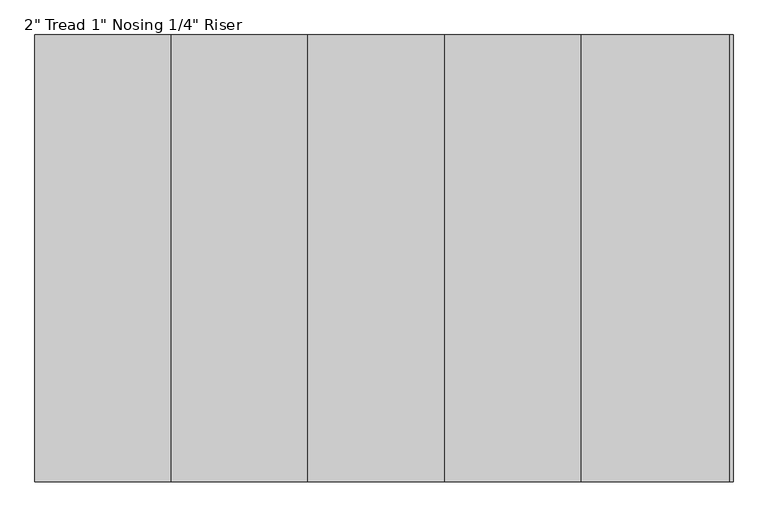
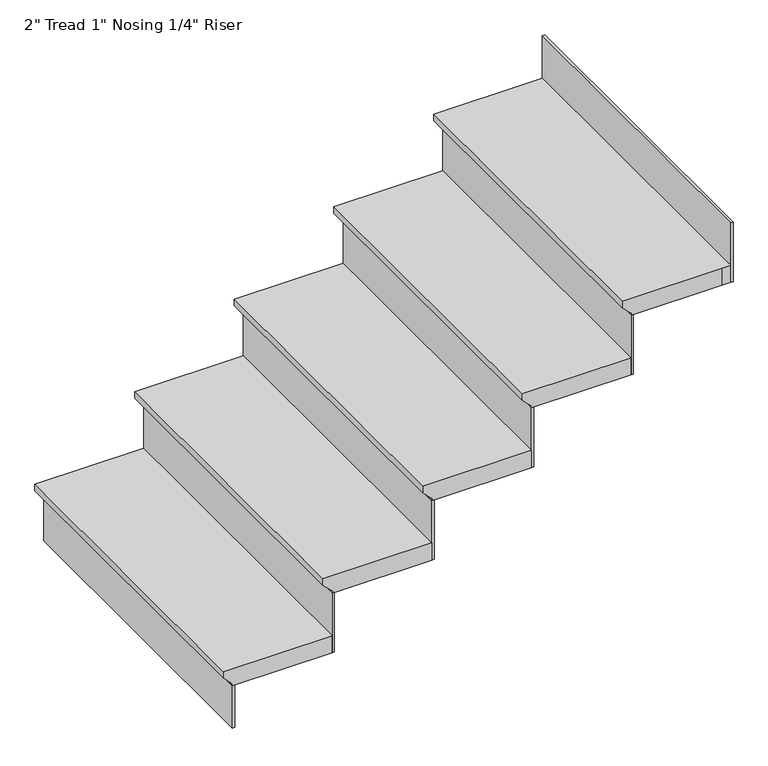
"""IFC4 building model written with IfcOpenShell, lengths in millimetres: stair flight geometry."""

from ifc_helpers import new_model, si_unit, origin, place, context, project, spatial, faceted_brep, source, transform, mapped, element, save


def stair_flight_54ffcc7a(model_context):
    return source(origin(), model_context, "Body", "Brep", [
        faceted_brep([(7509.0423568, -10720.6073314, 157.4131579), (7509.0423568, -10720.6073314, 176.4631579), (7509.0423568, -9806.2073314, 176.4631579), (7509.0423568, -9806.2073314, 157.4131579), (7534.4423568, -10720.6073314, 132.0131579), (7534.4423568, -9806.2073314, 132.0131579), (7813.8423568, -10720.6073314, 176.4631579), (7813.8423568, -9806.2073314, 176.4631579), (7534.4423568, -9806.2073314, 125.6631579), (7813.8423568, -9806.2073314, 125.6631579), (7813.8423568, -10720.6073314, 125.6631579), (7534.4423568, -10720.6073314, 125.6631579)], [[[0, 1, 2, 3]], [[4, 0, 3, 5]], [[2, 1, 6, 7]], [[8, 9, 10, 11]], [[2, 7, 9, 8, 5, 3]], [[8, 11, 4, 5]], [[6, 1, 0, 4, 11, 10]], [[7, 6, 10, 9]]]),
        faceted_brep([(7534.4423568, -10720.6073314, 125.6631579), (7534.4423568, -10720.6073314, 0.0), (7540.7923568, -10720.6073314, 0.0), (7540.7923568, -10720.6073314, 125.6631579), (7534.4423568, -9806.2073314, 125.6631579), (7540.7923568, -9806.2073314, 125.6631579), (7540.7923568, -9806.2073314, 0.0), (7534.4423568, -9806.2073314, 0.0)], [[[0, 1, 2, 3]], [[4, 5, 6, 7]], [[1, 0, 4, 7]], [[2, 1, 7, 6]], [[3, 2, 6, 5]], [[0, 3, 5, 4]]]),
        faceted_brep([(7813.8423568, -10720.6073314, 302.1263158), (7813.8423568, -10720.6073314, 125.6631579), (7820.1923568, -10720.6073314, 125.6631579), (7820.1923568, -10720.6073314, 302.1263158), (7813.8423568, -9806.2073314, 302.1263158), (7820.1923568, -9806.2073314, 302.1263158), (7820.1923568, -9806.2073314, 125.6631579), (7813.8423568, -9806.2073314, 125.6631579)], [[[0, 1, 2, 3]], [[4, 5, 6, 7]], [[1, 0, 4, 7]], [[2, 1, 7, 6]], [[3, 2, 6, 5]], [[0, 3, 5, 4]]]),
        faceted_brep([(7788.4423568, -9806.2073314, 352.9263158), (7788.4423568, -10720.6073314, 352.9263158), (8093.2423568, -10720.6073314, 352.9263158), (8093.2423568, -9806.2073314, 352.9263158), (7813.8423568, -9806.2073314, 302.1263158), (8093.2423568, -9806.2073314, 302.1263158), (8093.2423568, -10720.6073314, 302.1263158), (7813.8423568, -10720.6073314, 302.1263158), (7813.8423568, -9806.2073314, 308.4763158), (7788.4423568, -9806.2073314, 333.8763158), (7813.8423568, -10720.6073314, 308.4763158), (7788.4423568, -10720.6073314, 333.8763158)], [[[0, 1, 2, 3]], [[4, 5, 6, 7]], [[0, 3, 5, 4, 8, 9]], [[4, 7, 10, 8]], [[2, 1, 11, 10, 7, 6]], [[3, 2, 6, 5]], [[11, 1, 0, 9]], [[10, 11, 9, 8]]]),
        faceted_brep([(8093.2423568, -10720.6073314, 478.5894737), (8093.2423568, -10720.6073314, 302.1263158), (8099.5923568, -10720.6073314, 302.1263158), (8099.5923568, -10720.6073314, 478.5894737), (8093.2423568, -9806.2073314, 478.5894737), (8099.5923568, -9806.2073314, 478.5894737), (8099.5923568, -9806.2073314, 302.1263158), (8093.2423568, -9806.2073314, 302.1263158)], [[[0, 1, 2, 3]], [[4, 5, 6, 7]], [[1, 0, 4, 7]], [[2, 1, 7, 6]], [[3, 2, 6, 5]], [[0, 3, 5, 4]]]),
        faceted_brep([(8067.8423568, -9806.2073314, 529.3894737), (8067.8423568, -10720.6073314, 529.3894737), (8372.6423568, -10720.6073314, 529.3894737), (8372.6423568, -9806.2073314, 529.3894737), (8093.2423568, -9806.2073314, 478.5894737), (8372.6423568, -9806.2073314, 478.5894737), (8372.6423568, -10720.6073314, 478.5894737), (8093.2423568, -10720.6073314, 478.5894737), (8093.2423568, -9806.2073314, 484.9394737), (8067.8423568, -9806.2073314, 510.3394737), (8093.2423568, -10720.6073314, 484.9394737), (8067.8423568, -10720.6073314, 510.3394737)], [[[0, 1, 2, 3]], [[4, 5, 6, 7]], [[0, 3, 5, 4, 8, 9]], [[4, 7, 10, 8]], [[2, 1, 11, 10, 7, 6]], [[3, 2, 6, 5]], [[11, 1, 0, 9]], [[10, 11, 9, 8]]]),
        faceted_brep([(8372.6423568, -10720.6073314, 655.0526316), (8372.6423568, -10720.6073314, 478.5894737), (8378.9923568, -10720.6073314, 478.5894737), (8378.9923568, -10720.6073314, 655.0526316), (8372.6423568, -9806.2073314, 655.0526316), (8378.9923568, -9806.2073314, 655.0526316), (8378.9923568, -9806.2073314, 478.5894737), (8372.6423568, -9806.2073314, 478.5894737)], [[[0, 1, 2, 3]], [[4, 5, 6, 7]], [[1, 0, 4, 7]], [[2, 1, 7, 6]], [[3, 2, 6, 5]], [[0, 3, 5, 4]]]),
        faceted_brep([(8347.2423568, -9806.2073314, 705.8526316), (8347.2423568, -10720.6073314, 705.8526316), (8652.0423568, -10720.6073314, 705.8526316), (8652.0423568, -9806.2073314, 705.8526316), (8372.6423568, -9806.2073314, 655.0526316), (8652.0423568, -9806.2073314, 655.0526316), (8652.0423568, -10720.6073314, 655.0526316), (8372.6423568, -10720.6073314, 655.0526316), (8372.6423568, -9806.2073314, 661.4026316), (8347.2423568, -9806.2073314, 686.8026316), (8372.6423568, -10720.6073314, 661.4026316), (8347.2423568, -10720.6073314, 686.8026316)], [[[0, 1, 2, 3]], [[4, 5, 6, 7]], [[0, 3, 5, 4, 8, 9]], [[4, 7, 10, 8]], [[2, 1, 11, 10, 7, 6]], [[3, 2, 6, 5]], [[11, 1, 0, 9]], [[10, 11, 9, 8]]]),
        faceted_brep([(8931.4423568, -10720.6073314, 1007.9789474), (8931.4423568, -10720.6073314, 831.5157895), (8937.7923568, -10720.6073314, 831.5157895), (8937.7923568, -10720.6073314, 1007.9789474), (8931.4423568, -9806.2073314, 1007.9789474), (8937.7923568, -9806.2073314, 1007.9789474), (8937.7923568, -9806.2073314, 831.5157895), (8931.4423568, -9806.2073314, 831.5157895)], [[[0, 1, 2, 3]], [[4, 5, 6, 7]], [[1, 0, 4, 7]], [[2, 1, 7, 6]], [[3, 2, 6, 5]], [[0, 3, 5, 4]]]),
        faceted_brep([(8652.0423568, -10720.6073314, 831.5157895), (8652.0423568, -10720.6073314, 655.0526316), (8658.3923568, -10720.6073314, 655.0526316), (8658.3923568, -10720.6073314, 831.5157895), (8652.0423568, -9806.2073314, 831.5157895), (8658.3923568, -9806.2073314, 831.5157895), (8658.3923568, -9806.2073314, 655.0526316), (8652.0423568, -9806.2073314, 655.0526316)], [[[0, 1, 2, 3]], [[4, 5, 6, 7]], [[1, 0, 4, 7]], [[2, 1, 7, 6]], [[3, 2, 6, 5]], [[0, 3, 5, 4]]]),
        faceted_brep([(8931.4423568, -9806.2073314, 882.3157895), (8906.0423568, -9806.2073314, 882.3157895), (8626.6423568, -9806.2073314, 882.3157895), (8626.6423568, -10720.6073314, 882.3157895), (8906.0423568, -10720.6073314, 882.3157895), (8931.4423568, -10720.6073314, 882.3157895), (8906.0423568, -9806.2073314, 831.5157895), (8931.4423568, -9806.2073314, 831.5157895), (8931.4423568, -10720.6073314, 831.5157895), (8906.0423568, -10720.6073314, 831.5157895), (8652.0423568, -10720.6073314, 831.5157895), (8652.0423568, -9806.2073314, 831.5157895), (8652.0423568, -9806.2073314, 837.8657895), (8626.6423568, -9806.2073314, 863.2657895), (8652.0423568, -10720.6073314, 837.8657895), (8626.6423568, -10720.6073314, 863.2657895)], [[[0, 1, 2, 3, 4, 5]], [[6, 7, 8, 9, 10, 11]], [[1, 0, 7, 6]], [[2, 1, 6, 11, 12, 13]], [[11, 10, 14, 12]], [[4, 3, 15, 14, 10, 9]], [[5, 4, 9, 8]], [[0, 5, 8, 7]], [[15, 3, 2, 13]], [[14, 15, 13, 12]]]),
    ])


if __name__ == "__main__":
    model = new_model("IFC4")
    model_context = context("Model", 3, world=origin())
    ifc_project = project(units=[si_unit("LENGTHUNIT", "METRE", prefix="MILLI")], contexts=[model_context])
    site = spatial("IfcSite", under=ifc_project)
    building = spatial("IfcBuilding", under=site)
    placement = place(None, origin())
    stair_flight_shape = stair_flight_54ffcc7a(model_context)
    element("IfcStairFlight", 1, ObjectType="2\" Tread 1\" Nosing 1/4\" Riser", at=placement, inside=building, context=model_context, shape_type="MappedRepresentation", body=[
        mapped(stair_flight_shape, transform((0.0, 0.0, 0.0), x_axis=(1.0, 0.0, 0.0), y_axis=(0.0, 1.0, 0.0), z_axis=(0.0, 0.0, 1.0))),
    ])
    save(model, "model.ifc")

# Revit data of these elements
# Element 1 (IfcStairFlight, "2\" Tread 1\" Nosing 1/4\" Riser")
#   Materials on its faces: "MARBLE STAIRS 6\""
# Materials
#   "MARBLE STAIRS 6\"": class "Generic", colour RGB 120 120 120, transparency 0, Cost = 0
